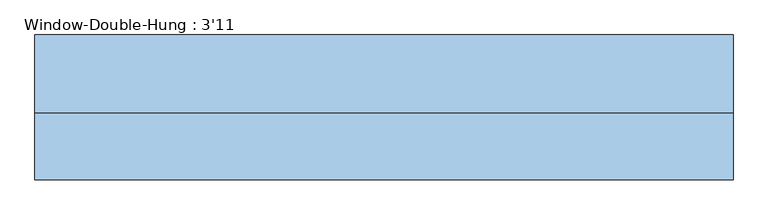
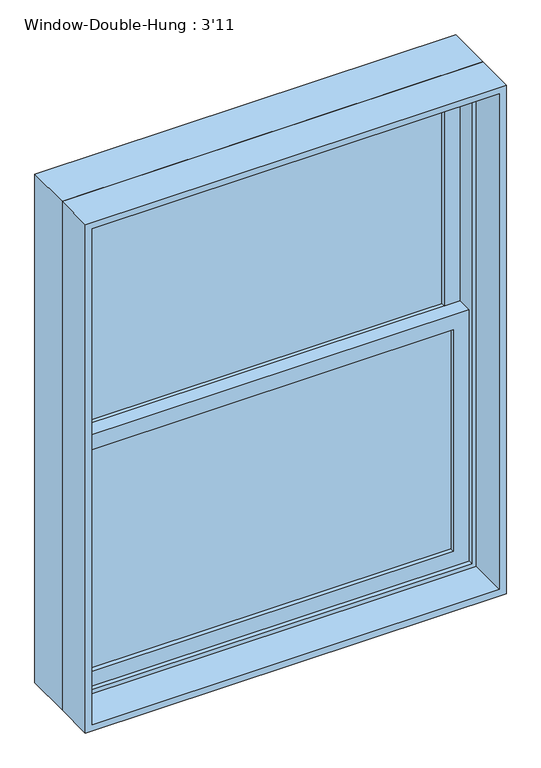
"""IFC4 building model written with IfcOpenShell, lengths in millimetres: window geometry, Window-Double-Hung : 3'11."""

from ifc_helpers import new_model, si_unit, frame, origin, place, context, project, spatial, polyline, outline, extrude, source, transform, mapped, element, save


def window_double_hung_3_11_b20011b0(model_context):
    return source(origin(), model_context, "Body", "SweptSolid", [
        extrude(outline(polyline([(520.7, 44.45), (520.7, 38.1), (-520.7, 38.1), (-520.7, 44.45), (520.7, 44.45)])), frame((0.0, 0.0, 990.6), z_axis=(0.0, 0.0, 1.0), x_axis=(1.0, 0.0, 0.0)), (0.0, 0.0, 1.0), 663.575),
        extrude(outline(polyline([(-520.7, 31.75), (520.7, 31.75), (520.7, 25.4), (-520.7, 25.4), (-520.7, 31.75)])), frame((0.0, 0.0, 990.6), z_axis=(0.0, 0.0, 1.0), x_axis=(1.0, 0.0, 0.0)), (0.0, 0.0, 1.0), 663.575),
        extrude(outline(polyline([(520.7, 88.9), (520.7, 82.55), (-520.7, 82.55), (-520.7, 88.9), (520.7, 88.9)])), frame((0.0, 0.0, 1698.625), z_axis=(0.0, 0.0, 1.0), x_axis=(1.0, 0.0, 0.0)), (0.0, 0.0, 1.0), 663.575),
        extrude(outline(polyline([(-520.7, 76.2), (520.7, 76.2), (520.7, 69.85), (-520.7, 69.85), (-520.7, 76.2)])), frame((0.0, 0.0, 1698.625), z_axis=(0.0, 0.0, 1.0), x_axis=(1.0, 0.0, 0.0)), (0.0, 0.0, 1.0), 663.575),
        extrude(outline(polyline([(1698.625, -565.15), (946.15, -565.15), (946.15, 565.15), (1698.625, 565.15), (1698.625, -565.15)]), holes=[polyline([(1654.175, 520.7), (990.6, 520.7), (990.6, -520.7), (1654.175, -520.7), (1654.175, 520.7)])]), frame((0.0, 12.7, 0.0), z_axis=(0.0, 1.0, 0.0), x_axis=(0.0, 0.0, 1.0)), (0.0, 0.0, 1.0), 44.45),
        extrude(outline(polyline([(2406.65, -565.15), (1654.175, -565.15), (1654.175, 565.15), (2406.65, 565.15), (2406.65, -565.15)]), holes=[polyline([(2362.2, 520.7), (1698.625, 520.7), (1698.625, -520.7), (2362.2, -520.7), (2362.2, 520.7)])]), frame((0.0, 57.15, 0.0), z_axis=(0.0, 1.0, 0.0), x_axis=(0.0, 0.0, 1.0)), (0.0, 0.0, 1.0), 44.45),
        extrude(outline(polyline([(2438.4, -596.9), (914.4, -596.9), (914.4, 596.9), (2438.4, 596.9), (2438.4, -596.9)]), holes=[polyline([(2406.65, 565.15), (946.15, 565.15), (946.15, -565.15), (2406.65, -565.15), (2406.65, 565.15)])]), frame((0.0, 0.0, 0.0), z_axis=(0.0, 1.0, 0.0), x_axis=(0.0, 0.0, 1.0)), (0.0, 0.0, 1.0), 133.35),
        extrude(outline(polyline([(2438.4, 596.9), (2438.4, -596.9), (914.4, -596.9), (914.4, 596.9), (2438.4, 596.9)]), holes=[polyline([(2419.35, 577.85), (933.45, 577.85), (933.45, -577.85), (2419.35, -577.85), (2419.35, 577.85)])]), frame((0.0, -114.3, 0.0), z_axis=(0.0, 1.0, 0.0), x_axis=(0.0, 0.0, 1.0)), (0.0, 0.0, 1.0), 114.3),
    ])


if __name__ == "__main__":
    model = new_model("IFC4")
    model_context = context("Model", 3, world=origin())
    ifc_project = project(units=[si_unit("LENGTHUNIT", "METRE", prefix="MILLI")], contexts=[model_context])
    site = spatial("IfcSite", under=ifc_project)
    building = spatial("IfcBuilding", under=site)
    placement = place(None, origin())
    window_double_hung_3_11_shape = window_double_hung_3_11_b20011b0(model_context)
    element("IfcWindow", 1, ObjectType="Window-Double-Hung : 3'11", at=placement, inside=building, context=model_context, shape_type="MappedRepresentation", body=[
        mapped(window_double_hung_3_11_shape, transform((0.0, 0.0, 0.0), x_axis=(1.0, 0.0, 0.0), y_axis=(0.0, 1.0, 0.0), z_axis=(0.0, 0.0, 1.0))),
    ])
    save(model, "model.ifc")

# Revit data of these elements
# Type "Window-Double-Hung : 3'11"
#   Type Mark = "21"
#   Fire Rating = "0.5h"
#   Construction Type Id = "DG-DR"
#   Assembly Code = "B2020100"
#   Analytic Construction = "Double glazing - domestic"
#   Wall Thickness [instance default] = 0' - 6"
#   Window Inset [instance default] = 0' - 0"
#   Visual Light Transmittance = 0.81
#   Thermal Resistance (R) = 1.8146 (h·ft²·°F)/BTU
#   Solar Heat Gain Coefficient = 0.76
#   Muntin Width = 3' - 5"
#   Muntin Height = 2' - 2 1/8"
#   Interior Wall Closure [instance default] = 0' - 1 1/2"
#   Rough Width = 3' - 11 1/2"
#   Rough Height = 5' - 0 1/2"
#   Frame Extension [instance default] = 0' - 1 1/4"
#   Exterior Wall Closure [instance default] = 0' - 0 1/2"
#   Extension Jamb [instance default] = 0' - 1 1/2"
#   Heat Transfer Coefficient (U) = 0.5511 BTU/(h·ft²·°F)
#   Height = 5' - 0"
#   Width = 3' - 11"
#   Top Muntin Visibility = yes
#   Indicator Visibility [instance default] = yes
#   Extension Jamb Visibility [instance default] = yes
#   Interior Trim Visibility [instance default] = yes
#   Exterior Trim Visibility [instance default] = yes
#   Define Thermal Properties by = 1
#   Bottom Muntin Visibility = yes
#   Muntin Pattern = Muntin Pattern_2x2 : Muntin Pattern_2x2
#   Interior Trim Material = Wood - Stained
#   Interior Trim = Trim-Window-Interior-Flat : Picture Frame
#   Exterior Trim Material = Clad - White
#   Exterior Trim = Trim-Window-Exterior-Flat : with Sill
#   Glass Panel Material = Glass
#   Exterior Frame Material = Clad - White
#   Interior Frame Material = Wood - Stained
#   Wall Closure = (empty or 0)
# Element 1 (IfcWindow, "Window-Double-Hung : 3'11")
#   Wall Thickness = 0' - 9"
#   Extension Jamb = 0' - 4 1/2"
#   Materials on its faces: "Wood - Stained", "Glass", "Clad - White"
# Materials
#   "Wood - Stained": class "Wood", colour RGB 224 178 126, transparency 0, Cost = 0
#   "Clad - White": class "Wood", colour RGB 242 242 238, transparency 0, Cost = 0
#   "Glass": class "Glass", colour RGB 154 182 205, transparency 0.85, Description = "Soda Lime Glass", Cost = 0
